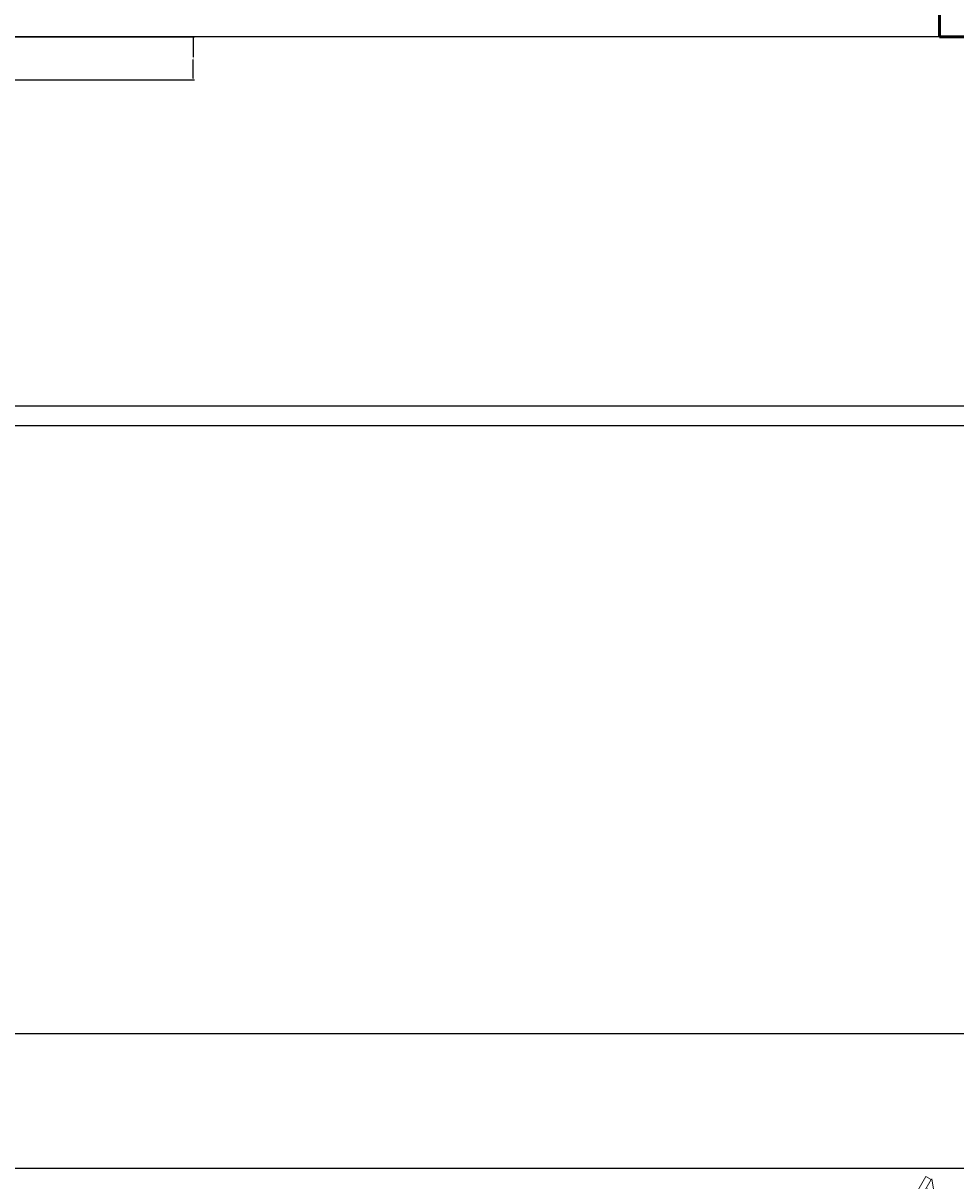
# Model space of a CAD drawing. Units: inches. Extents: x 1865 to 2541, y 1997 to 2759.
# Tile 7 of 11: x 2070 to 2200, y 2405 to 2566. Entities that reach past the tile are written whole.
import ezdxf

# ---------------------------------------------------------------- set-up
doc = ezdxf.new("R2010")
doc.units = ezdxf.units.IN
for name, color, linetype, lineweight in [('A-ANNO-DIMS', 2, 'Continuous', 18), ('A-WALL', 7, 'Continuous', 50), ('DINING TABLE', 120, 'Continuous', 13)]:
    doc.layers.add(name, color=color, linetype=linetype, lineweight=lineweight)
doc.styles.get("Standard").update_dxf_attribs({"font": 'arial.ttf'})
doc.dimstyles.get("Standard").update_dxf_attribs({"dimtxt": 0.18, "dimasz": 0.18, "dimexe": 0.18, "dimexo": 0.0625, "dimgap": 0.09, "dimtad": 0, "dimtih": 1, "dimtoh": 1, "dimdec": 4, "dimzin": 0, "dimdsep": 46, "dimtxsty": 'Standard', "dimcen": 0.09, "dimadec": 0, "dimazin": 0, "dimtfac": 1, "dimtdec": 4, "dimtofl": 0, "dimtmove": 0, "dimatfit": 3, "dimfxl": 1, "dimtolj": 1, "dimtzin": 0, "dimarcsym": 0})

# ---------------------------------------------------------------- blocks, each defined once
blk = doc.blocks.new('A$C45501D90')
for p, q in [((-242.2, 1133.5), (224, 1133.5)), ((-242.2, 1112.8), (-242.2, 1133.5)), ((224, 1112.8), (-242.2, 1112.8)), ((-242.2, 1111.2), (-202.3, 1079.2)), ((-203.9, 1106.4), (-165.6, 1108)), ((-168.8, 1080.8), (-203.9, 1106.4)), ((-165.6, 1108), (-167.2, 1085.6)), ((-156, 1109.6), (-132, 1085.6)), ((-119.3, 1085.6), (-143.2, 1108)), ((-143.2, 1108), (-133.6, 1108)), ((-133.6, 1108), (-122.5, 1098.4)), ((-122.5, 1098.4), (-119.3, 1101.6)), ((-119.3, 1101.6), (-117.7, 1087.2)), ((-108.1, 1109.6), (-84.1, 1085.6)), ((-71.4, 1085.6), (-95.3, 1108)), ((-95.3, 1108), (-85.7, 1108)), ((-85.7, 1108), (-74.6, 1098.4)), ((-74.6, 1098.4), (-71.4, 1101.6)), ((-71.4, 1101.6), (-69.8, 1087.2)), ((-60.2, 1109.6), (-36.2, 1085.6)), ((-23.5, 1085.6), (-47.4, 1108)), ((-47.4, 1108), (-37.8, 1108)), ((-37.8, 1108), (-26.7, 1098.4)), ((-26.7, 1098.4), (-23.5, 1101.6)), ((-23.5, 1101.6), (-21.9, 1087.2)), ((8.5, 1101.6), (6.9, 1087.2)), ((8.5, 1085.6), (32.4, 1108)), ((11.6, 1098.4), (8.5, 1101.6)), ((22.8, 1108), (11.6, 1098.4)), ((45.2, 1109.6), (21.2, 1085.6)), ((32.4, 1108), (22.8, 1108)), ((56.3, 1101.6), (54.8, 1087.2)), ((56.3, 1085.6), (80.3, 1108)), ((59.5, 1098.4), (56.3, 1101.6)), ((70.7, 1108), (59.5, 1098.4)), ((93.1, 1109.6), (69.1, 1085.6)), ((80.3, 1108), (70.7, 1108)), ((104.2, 1101.6), (102.6, 1087.2)), ((104.2, 1085.6), (128.2, 1108)), ((107.4, 1098.4), (104.2, 1101.6)), ((118.6, 1108), (107.4, 1098.4)), ((141, 1109.6), (117, 1085.6)), ((128.2, 1108), (118.6, 1108)), ((188.9, 1106.4), (150.5, 1108)), ((150.5, 1108), (152.1, 1085.6)), ((153.7, 1080.8), (188.9, 1106.4)), ((224, 1112.8), (187.3, 1079.2)), ((224, 1133.5), (224, 1112.8)), ((-197.3, 1061.6), (-238.9, 627.6)), ((-202.3, 1079.2), (-168.8, 1080.8)), ((161.8, 1076.1), (-181.4, 1076.1)), ((-132, 1085.6), (-119.3, 1085.6)), ((-84.1, 1085.6), (-71.4, 1085.6)), ((-36.2, 1085.6), (-23.5, 1085.6)), ((21.2, 1085.6), (8.5, 1085.6)), ((69.1, 1085.6), (56.3, 1085.6)), ((117, 1085.6), (104.2, 1085.6)), ((187.3, 1079.2), (153.7, 1080.8)), ((225.2, 627.8), (177.6, 1061.8)), ((842.6, 766.1), (860.5, 776.5)), ((860.5, 776.5), (1093.6, 372.8)), ((-1102.7, 357), (-869.7, 760.7)), ((-851.7, 750.4), (-1084.8, 346.6)), ((-869.7, 760.7), (-851.7, 750.4)), ((-848.7, 752.3), (-841, 701.8)), ((841.2, 765.3), (833.5, 714.8)), ((1075.7, 362.4), (842.6, 766.1)), ((-863.7, 716.7), (-884.3, 684.4)), ((-859.2, 673.6), (-863.7, 716.7)), ((-841, 701.8), (-859.2, 673.6)), ((820.7, 701.7), (424.1, 520.7)), ((833.5, 714.8), (851.7, 686.6)), ((1012.8, 397.9), (841.2, 695.1)), ((851.7, 686.6), (856.2, 729.8)), ((856.2, 729.8), (876.7, 697.4)), ((876.7, 697.4), (856.6, 687.6)), ((-851, 678.1), (-1022.6, 380.9)), ((-895.4, 665), (-900.2, 656.7)), ((-900.2, 656.7), (-897.5, 642.2)), ((-888.1, 633.1), (-895.4, 665)), ((-890.4, 676.9), (-881.7, 644.2)), ((-884.3, 684.4), (-864.1, 674.6)), ((-431.1, 509), (-830.8, 684.8)), ((882.9, 689.9), (874.2, 657.2)), ((874.2, 657.2), (880.6, 646.1)), ((880.6, 646.1), (887.9, 678)), ((894.4, 654.1), (882.7, 645.5)), ((887.9, 678), (892.7, 669.7)), ((892.7, 669.7), (890, 655.2)), ((890, 655.2), (894.4, 654.1)), ((-919.4, 623.5), (-924.2, 615.2)), ((-924.2, 615.2), (-921.5, 600.8)), ((-912, 591.6), (-919.4, 623.5)), ((-914.4, 635.4), (-905.6, 602.7)), ((-897.5, 642.2), (-901.9, 641.1)), ((-901.9, 641.1), (-890.2, 632.5)), ((-881.7, 644.2), (-888.1, 633.1)), ((906.9, 648.4), (898.1, 615.7)), ((898.1, 615.7), (904.5, 604.6)), ((904.5, 604.6), (911.9, 636.5)), ((918.3, 612.6), (906.7, 604)), ((911.9, 636.5), (916.7, 628.2)), ((916.7, 628.2), (914, 613.8)), ((914, 613.8), (918.3, 612.6)), ((-943.3, 582), (-948.1, 573.8)), ((-948.1, 573.8), (-945.4, 559.3)), ((-936, 550.1), (-943.3, 582)), ((-938.3, 593.9), (-929.6, 561.2)), ((-921.5, 600.8), (-925.8, 599.6)), ((-925.8, 599.6), (-914.2, 591)), ((-905.6, 602.7), (-912, 591.6)), ((-223, 610.1), (209.4, 610.1)), ((930.8, 606.9), (922.1, 574.2)), ((922.1, 574.2), (928.4, 563.1)), ((928.4, 563.1), (935.8, 595.1)), ((942.3, 571.1), (930.6, 562.6)), ((935.8, 595.1), (940.6, 586.8)), ((940.6, 586.8), (937.9, 572.3)), ((937.9, 572.3), (942.3, 571.1)), ((-964.6, 526.1), (-965.7, 530.5)), ((-965.7, 530.5), (-952.5, 524.7)), ((-945.4, 559.3), (-949.8, 558.1)), ((-949.8, 558.1), (-938.1, 549.6)), ((-929.6, 561.2), (-936, 550.1)), ((950.8, 524.4), (944.4, 535.5)), ((944.4, 535.5), (975.7, 525.9)), ((958.2, 543.5), (945, 537.7)), ((957.1, 539.1), (958.2, 543.5)), ((970.9, 534.2), (957.1, 539.1)), ((975.7, 525.9), (970.9, 534.2)), ((-991, 502.7), (-958.3, 511.4)), ((-951.9, 522.5), (-983.2, 512.9)), ((-983.2, 512.9), (-978.5, 521.2)), ((-978.5, 521.2), (-964.6, 526.1)), ((-958.3, 511.4), (-951.9, 522.5)), ((-5.6, 508.7, 90.8), (0.4, 508.7, 90.8)), ((-5.6, 317.7, 90.8), (-5.6, 508.7, 90.8)), ((0.4, 508.7, 90.8), (0.4, 317.7, 90.8)), ((5.8, 317.7, 90.8), (5.8, 508.7, 90.8)), ((5.8, 508.7, 90.8), (11.8, 508.7, 90.8)), ((11.8, 508.7, 90.8), (11.8, 317.7, 90.8)), ((416.9, 498.2), (633.1, 123.7)), ((983.5, 515.7), (950.8, 524.4)), ((968.4, 494), (999.7, 484.4)), ((974.7, 483), (968.4, 494)), ((982.2, 502), (968.9, 496.2)), ((981, 497.6), (982.2, 502)), ((994.9, 492.7), (981, 497.6)), ((999.7, 484.4), (994.9, 492.7)), ((-1015, 461.2), (-982.3, 469.9)), ((-975.9, 481), (-1007.2, 471.4)), ((-1007.2, 471.4), (-1002.4, 479.7)), ((-1002.4, 479.7), (-988.5, 484.6)), ((-988.5, 484.6), (-989.7, 489)), ((-989.7, 489), (-976.5, 483.2)), ((-982.3, 469.9), (-975.9, 481)), ((-639.9, 111.9), (-423.7, 486.4)), ((1007.4, 474.2), (974.7, 483)), ((998.7, 441.5), (992.3, 452.5)), ((992.3, 452.5), (1023.6, 443)), ((1006.1, 460.5), (992.9, 454.7)), ((1005, 456.2), (1006.1, 460.5)), ((1018.8, 451.3), (1005, 456.2)), ((1023.6, 443), (1018.8, 451.3)), ((-1060.1, 376.6), (-1042.3, 410.6)), ((-1042.3, 410.6), (-1023.8, 398.1)), ((-1038.9, 419.7), (-1006.2, 428.5)), ((-999.8, 439.5), (-1031.1, 430)), ((-1031.1, 430), (-1026.3, 438.3)), ((-1026.3, 438.3), (-1012.5, 443.1)), ((-1012.5, 443.1), (-1013.6, 447.5)), ((-1013.6, 447.5), (-1000.4, 441.7)), ((-1006.2, 428.5), (-999.8, 439.5)), ((1031.4, 432.7), (998.7, 441.5)), ((1034.8, 423.6), (1016.3, 411.1)), ((1052.6, 389.6), (1034.8, 423.6)), ((-1020.4, 394.3), (-1060.1, 376.6)), ((-1035.8, 364.4), (-1020.4, 394.3)), ((656.3, 118.9), (1008.4, 377.1)), ((1028.3, 377.5), (1012.9, 407.3)), ((1012.9, 407.3), (1052.6, 389.6)), ((1075.9, 358.8), (1028.3, 377.5)), ((1093.6, 372.8), (1075.7, 362.4)), ((-1084.8, 346.6), (-1102.7, 357)), ((-1083.4, 345.8), (-1035.8, 364.4)), ((-1018, 360), (-663, 106.9)), ((-22.3, 329.1, 90.8), (-22.3, 344.6, 90.8)), ((-22.3, 344.6, 90.8), (-5.6, 344.6, 90.8)), ((-5.6, 329.1, 90.8), (-22.3, 329.1, 90.8)), ((0.4, 344.6, 90.8), (5.8, 344.6, 90.8)), ((5.8, 329.1, 90.8), (0.4, 329.1, 90.8)), ((11.8, 344.6, 90.8), (27.3, 344.6, 90.8)), ((27.3, 329.1, 90.8), (11.8, 329.1, 90.8)), ((27.3, 344.6, 90.8), (27.3, 329.1, 90.8)), ((-175.3, 276.1, 90.8), (-104.8, 293.2, 90.8)), ((-104.8, 293.2, 90.8), (-85.5, 278.4, 90.8)), ((-85.5, 278.4, 90.8), (-52.1, 293.9, 90.8)), ((-52.1, 293.9, 90.8), (9.5, 276.1, 90.8)), ((0.4, 317.7, 90.8), (-5.6, 317.7, 90.8)), ((11.8, 317.7, 90.8), (5.8, 317.7, 90.8)), ((134.3, 288, 90.8), (184.3, 235.5, 90.8)), ((149.7, 213.9, 90.8), (134.3, 288, 90.8)), ((-436.3, 265.3, 90.8), (-433.3, 270.5, 90.8)), ((-270.9, 169.9, 90.8), (-436.3, 265.3, 90.8)), ((-433.3, 270.5, 90.8), (-267.9, 175, 90.8)), ((-430.6, 275.2, 90.8), (-427.6, 280.3, 90.8)), ((-265.2, 179.7, 90.8), (-430.6, 275.2, 90.8)), ((-427.6, 280.3, 90.8), (-262.3, 184.9, 90.8)), ((-103.3, 252.4, 90.8), (-175.3, 276.1, 90.8)), ((-59.5, 246.5, 90.8), (-103.3, 252.4, 90.8)), ((9.5, 276.1, 90.8), (-59.5, 246.5, 90.8)), ((255.2, 161.9, 90.8), (420.6, 257.3, 90.8)), ((423.5, 252.2, 90.8), (258.2, 156.7, 90.8)), ((260.9, 152, 90.8), (426.2, 247.5, 90.8)), ((420.6, 257.3, 90.8), (423.5, 252.2, 90.8)), ((426.2, 247.5, 90.8), (429.2, 242.3, 90.8)), ((-285.5, 198.3, 90.8), (-277.8, 211.7, 90.8)), ((-277.8, 211.7, 90.8), (-264.3, 204, 90.8)), ((-264.3, 204, 90.8), (-272.1, 190.5, 90.8)), ((166.5, 173, 90.8), (149.7, 213.9, 90.8)), ((184.3, 235.5, 90.8), (181.1, 211.4, 90.8)), ((181.1, 211.4, 90.8), (211.3, 190.3, 90.8)), ((429.2, 242.3, 90.8), (263.8, 146.9, 90.8)), ((-302.5, 168.8, 90.8), (-294.2, 183.3, 90.8)), ((-289.1, 161.1, 90.8), (-302.5, 168.8, 90.8)), ((-291.2, 188.5, 90.8), (-288.5, 193.1, 90.8)), ((-280.7, 175.5, 90.8), (-289.1, 161.1, 90.8)), ((-275.1, 185.4, 90.8), (-277.8, 180.7, 90.8)), ((-267.9, 175, 90.8), (-270.9, 169.9, 90.8)), ((-262.3, 184.9, 90.8), (-265.2, 179.7, 90.8)), ((226.7, 128.1, 90.8), (166.5, 173, 90.8)), ((211.3, 190.3, 90.8), (226.7, 128.1, 90.8)), ((256.6, 182, 90.8), (270.1, 189.8, 90.8)), ((265, 167.5, 90.8), (256.6, 182, 90.8)), ((270.1, 189.8, 90.8), (278.4, 175.3, 90.8)), ((281.4, 170.1, 90.8), (284.1, 165.5, 90.8)), ((-273.6, 117.6, 90.8), (-227.4, 162.1, 90.8)), ((-227.4, 162.1, 90.8), (-236.2, 87.5, 90.8)), ((258.2, 156.7, 90.8), (255.2, 161.9, 90.8)), ((263.8, 146.9, 90.8), (260.9, 152, 90.8)), ((270.7, 157.7, 90.8), (268, 162.4, 90.8)), ((281.4, 139.1, 90.8), (273.7, 152.5, 90.8)), ((294.9, 146.8, 90.8), (281.4, 139.1, 90.8)), ((287.1, 160.3, 90.8), (294.9, 146.8, 90.8)), ((-276.8, 80.9, 90.8), (-273.6, 117.6, 90.8)), ((-236.2, 87.5, 90.8), (-263.2, 52.5, 90.8)), ((-319.8, 2.1, 90.8), (-299.3, 71.7, 90.8)), ((-263.2, 52.5, 90.8), (-319.8, 2.1, 90.8)), ((-299.3, 71.7, 90.8), (-276.8, 80.9, 90.8)), ((242.9, -24.6, 90.8), (299.4, 25.9, 90.8)), ((299.4, 25.9, 90.8), (278.9, -43.7, 90.8)), ((215.8, -59.5, 90.8), (242.9, -24.6, 90.8)), ((207, -134.1, 90.8), (215.8, -59.5, 90.8)), ((256.4, -53, 90.8), (253.2, -89.7, 90.8)), ((278.9, -43.7, 90.8), (256.4, -53, 90.8)), ((-656.3, -118.9), (-1008.4, -377.1)), ((-449.6, -214.4, 90.8), (-284.2, -118.9, 90.8)), ((-315.2, -118.9, 90.8), (-301.8, -111.1, 90.8)), ((-307.5, -132.3, 90.8), (-315.2, -118.9, 90.8)), ((-301.8, -111.1, 90.8), (-294, -124.6, 90.8)), ((-284.2, -118.9, 90.8), (-281.2, -124.1, 90.8)), ((-247, -100.1, 90.8), (-186.8, -145, 90.8)), ((-231.7, -162.3, 90.8), (-247, -100.1, 90.8)), ((253.2, -89.7, 90.8), (207, -134.1, 90.8)), ((639.9, -111.9), (423.7, -486.4)), ((1018, -360), (663, -106.9)), ((-416.9, -498.2), (-633.1, -123.7)), ((-281.2, -124.1, 90.8), (-446.6, -219.5, 90.8)), ((-443.9, -224.2, 90.8), (-278.5, -128.7, 90.8)), ((-275.5, -133.9, 90.8), (-440.9, -229.4, 90.8)), ((-301.8, -142.1, 90.8), (-304.5, -137.5, 90.8)), ((-290.4, -161.8, 90.8), (-298.8, -147.3, 90.8)), ((-291, -129.7, 90.8), (-288.3, -134.4, 90.8)), ((-277, -154, 90.8), (-290.4, -161.8, 90.8)), ((-285.4, -139.5, 90.8), (-277, -154, 90.8)), ((-278.5, -128.7, 90.8), (-275.5, -133.9, 90.8)), ((-201.5, -183.4, 90.8), (-231.7, -162.3, 90.8)), ((-186.8, -145, 90.8), (-170.1, -185.9, 90.8)), ((241.9, -156.9, 90.8), (244.9, -151.7, 90.8)), ((407.3, -252.4, 90.8), (241.9, -156.9, 90.8)), ((244, -176, 90.8), (251.7, -162.5, 90.8)), ((244.9, -151.7, 90.8), (410.3, -247.2, 90.8)), ((247.6, -147.1, 90.8), (250.6, -141.9, 90.8)), ((413, -242.5, 90.8), (247.6, -147.1, 90.8)), ((250.6, -141.9, 90.8), (415.9, -237.4, 90.8)), ((254.7, -157.4, 90.8), (257.4, -152.7, 90.8)), ((260.4, -147.6, 90.8), (268.7, -133.1, 90.8)), ((270.8, -160.5, 90.8), (268.1, -165.1, 90.8)), ((268.7, -133.1, 90.8), (282.2, -140.8, 90.8)), ((282.2, -140.8, 90.8), (273.8, -155.3, 90.8)), ((-204.7, -207.6, 90.8), (-201.5, -183.4, 90.8)), ((-170.1, -185.9, 90.8), (-154.7, -260.1, 90.8)), ((257.4, -183.7, 90.8), (244, -176, 90.8)), ((265.2, -170.3, 90.8), (257.4, -183.7, 90.8)), ((-446.6, -219.5, 90.8), (-449.6, -214.4, 90.8)), ((-440.9, -229.4, 90.8), (-443.9, -224.2, 90.8)), ((-154.7, -260.1, 90.8), (-204.7, -207.6, 90.8)), ((-29.8, -248.2, 90.8), (39.2, -218.5, 90.8)), ((39.2, -218.5, 90.8), (83, -224.4, 90.8)), ((83, -224.4, 90.8), (154.9, -248.2, 90.8)), ((415.9, -237.4, 90.8), (413, -242.5, 90.8)), ((31.8, -266, 90.8), (-29.8, -248.2, 90.8)), ((65.2, -250.4, 90.8), (31.8, -266, 90.8)), ((84.4, -265.2, 90.8), (65.2, -250.4, 90.8)), ((154.9, -248.2, 90.8), (84.4, -265.2, 90.8)), ((410.3, -247.2, 90.8), (407.3, -252.4, 90.8)), ((-47.6, -316.6, 90.8), (-47.6, -301.1, 90.8)), ((-47.6, -301.1, 90.8), (-32.1, -301.1, 90.8)), ((-32.1, -316.6, 90.8), (-47.6, -316.6, 90.8)), ((-32.1, -480.7, 90.8), (-32.1, -289.8, 90.8)), ((-32.1, -289.8, 90.8), (-26.1, -289.8, 90.8)), ((-26.1, -289.8, 90.8), (-26.1, -480.7, 90.8)), ((-26.1, -301.1, 90.8), (-20.8, -301.1, 90.8)), ((-20.8, -316.6, 90.8), (-26.1, -316.6, 90.8)), ((-20.8, -480.7, 90.8), (-20.8, -289.8, 90.8)), ((-20.8, -289.8, 90.8), (-14.8, -289.8, 90.8)), ((-14.8, -289.8, 90.8), (-14.8, -480.7, 90.8)), ((-14.8, -301.1, 90.8), (1.9, -301.1, 90.8)), ((1.9, -316.6, 90.8), (-14.8, -316.6, 90.8)), ((1.9, -301.1, 90.8), (1.9, -316.6, 90.8)), ((-1093.6, -372.8), (-1075.7, -362.4)), ((-1075.9, -358.8), (-1028.3, -377.5)), ((-1075.7, -362.4), (-842.6, -766.1)), ((851.7, -750.4), (1084.8, -346.6)), ((1102.7, -357), (869.7, -760.7)), ((1035.8, -364.4), (1020.4, -394.3)), ((1083.4, -345.8), (1035.8, -364.4)), ((1084.8, -346.6), (1102.7, -357)), ((-860.5, -776.5), (-1093.6, -372.8)), ((-1052.6, -389.6), (-1034.8, -423.6)), ((-1012.9, -407.3), (-1052.6, -389.6)), ((-1028.3, -377.5), (-1012.9, -407.3)), ((-1012.8, -397.9), (-841.2, -695.1)), ((851, -678.1), (1022.6, -380.9)), ((1020.4, -394.3), (1060.1, -376.6)), ((1042.3, -410.6), (1023.8, -398.1)), ((1060.1, -376.6), (1042.3, -410.6)), ((-1034.8, -423.6), (-1016.3, -411.1)), ((-1031.4, -432.7), (-998.7, -441.5)), ((-1023.6, -443), (-1018.8, -451.3)), ((-992.3, -452.5), (-1023.6, -443)), ((-998.7, -441.5), (-992.3, -452.5)), ((1006.2, -428.5), (999.8, -439.5)), ((999.8, -439.5), (1031.1, -430)), ((1013.6, -447.5), (1000.4, -441.7)), ((1038.9, -419.7), (1006.2, -428.5)), ((1026.3, -438.3), (1012.5, -443.1)), ((1012.5, -443.1), (1013.6, -447.5)), ((1031.1, -430), (1026.3, -438.3)), ((-1018.8, -451.3), (-1005, -456.2)), ((-1007.4, -474.2), (-974.7, -483)), ((-1006.1, -460.5), (-992.9, -454.7)), ((-1005, -456.2), (-1006.1, -460.5)), ((-968.4, -494), (-999.7, -484.4)), ((-999.7, -484.4), (-994.9, -492.7)), ((-974.7, -483), (-968.4, -494)), ((-26.1, -480.7, 90.8), (-32.1, -480.7, 90.8)), ((-14.8, -480.7, 90.8), (-20.8, -480.7, 90.8)), ((982.3, -469.9), (975.9, -481)), ((975.9, -481), (1007.2, -471.4)), ((989.7, -489), (976.5, -483.2)), ((1015, -461.2), (982.3, -469.9)), ((1002.4, -479.7), (988.5, -484.6)), ((988.5, -484.6), (989.7, -489)), ((1007.2, -471.4), (1002.4, -479.7)), ((-994.9, -492.7), (-981, -497.6)), ((-983.5, -515.7), (-950.8, -524.4)), ((-982.2, -502), (-968.9, -496.2)), ((-981, -497.6), (-982.2, -502)), ((-944.4, -535.5), (-975.7, -525.9)), ((-975.7, -525.9), (-970.9, -534.2)), ((-950.8, -524.4), (-944.4, -535.5)), ((-820.7, -701.7), (-424.1, -520.7)), ((431.1, -509), (830.8, -684.8)), ((958.3, -511.4), (951.9, -522.5)), ((951.9, -522.5), (983.2, -512.9)), ((965.7, -530.5), (952.5, -524.7)), ((991, -502.7), (958.3, -511.4)), ((978.5, -521.2), (964.6, -526.1)), ((964.6, -526.1), (965.7, -530.5)), ((983.2, -512.9), (978.5, -521.2)), ((-970.9, -534.2), (-957.1, -539.1)), ((-958.2, -543.5), (-945, -537.7)), ((-957.1, -539.1), (-958.2, -543.5)), ((-942.3, -571.1), (-930.6, -562.6)), ((-928.4, -563.1), (-935.8, -595.1)), ((-922.1, -574.2), (-928.4, -563.1)), ((929.6, -561.2), (936, -550.1)), ((938.3, -593.9), (929.6, -561.2)), ((936, -550.1), (943.3, -582)), ((949.8, -558.1), (938.1, -549.6)), ((945.4, -559.3), (949.8, -558.1)), ((948.1, -573.8), (945.4, -559.3)), ((-937.9, -572.3), (-942.3, -571.1)), ((-940.6, -586.8), (-937.9, -572.3)), ((-935.8, -595.1), (-940.6, -586.8)), ((-930.8, -606.9), (-922.1, -574.2)), ((-918.3, -612.6), (-906.7, -604)), ((-904.5, -604.6), (-911.9, -636.5)), ((-898.1, -615.7), (-904.5, -604.6)), ((218.9, -611.6), (-213.5, -611.6)), ((223, -610.1), (-209.4, -610.1)), ((905.6, -602.7), (912, -591.6)), ((914.4, -635.4), (905.6, -602.7)), ((912, -591.6), (919.4, -623.5)), ((925.8, -599.6), (914.2, -591)), ((921.5, -600.8), (925.8, -599.6)), ((924.2, -615.2), (921.5, -600.8)), ((943.3, -582), (948.1, -573.8)), ((-914, -613.8), (-918.3, -612.6)), ((-916.7, -628.2), (-914, -613.8)), ((-911.9, -636.5), (-916.7, -628.2)), ((-906.9, -648.4), (-898.1, -615.7)), ((-894.4, -654.1), (-882.7, -645.5)), ((-880.6, -646.1), (-887.9, -678)), ((-874.2, -657.2), (-880.6, -646.1)), ((-229.3, -629.3), (-181.8, -1063.3)), ((-225.2, -627.8), (-177.6, -1061.8)), ((193.2, -1063.1), (234.8, -629.1)), ((197.3, -1061.6), (238.9, -627.6)), ((881.7, -644.2), (888.1, -633.1)), ((890.4, -676.9), (881.7, -644.2)), ((888.1, -633.1), (895.4, -665)), ((901.9, -641.1), (890.2, -632.5)), ((897.5, -642.2), (901.9, -641.1)), ((900.2, -656.7), (897.5, -642.2)), ((919.4, -623.5), (924.2, -615.2)), ((-890, -655.2), (-894.4, -654.1)), ((-892.7, -669.7), (-890, -655.2)), ((-887.9, -678), (-892.7, -669.7)), ((-882.9, -689.9), (-874.2, -657.2)), ((-876.7, -697.4), (-856.6, -687.6)), ((-851.7, -686.6), (-856.2, -729.8)), ((-833.5, -714.8), (-851.7, -686.6)), ((841, -701.8), (859.2, -673.6)), ((859.2, -673.6), (863.7, -716.7)), ((863.7, -716.7), (884.3, -684.4)), ((884.3, -684.4), (864.1, -674.6)), ((895.4, -665), (900.2, -656.7)), ((-856.2, -729.8), (-876.7, -697.4)), ((-841.2, -765.3), (-833.5, -714.8)), ((848.7, -752.3), (841, -701.8)), ((-842.6, -766.1), (-860.5, -776.5)), ((869.7, -760.7), (851.7, -750.4)), ((-231.3, -1112.7), (-191.4, -1080.8)), ((-227.2, -1111.2), (-187.3, -1079.2)), ((-157.9, -1082.4), (-193, -1107.9)), ((-191.4, -1080.8), (-157.9, -1082.4)), ((-153.7, -1080.8), (-188.9, -1106.4)), ((-187.3, -1079.2), (-153.7, -1080.8)), ((-165.9, -1077.6), (177.3, -1077.6)), ((-161.8, -1076.1), (181.4, -1076.1)), ((-154.7, -1109.5), (-156.3, -1087.1)), ((-150.5, -1108), (-152.1, -1085.6)), ((-145.1, -1111.1), (-121.1, -1087.1)), ((-141, -1109.6), (-117, -1085.6)), ((-108.4, -1087.1), (-132.3, -1109.5)), ((-104.2, -1085.6), (-128.2, -1108)), ((-122.7, -1109.5), (-111.6, -1099.9)), ((-121.1, -1087.1), (-108.4, -1087.1)), ((-118.6, -1108), (-107.4, -1098.4)), ((-117, -1085.6), (-104.2, -1085.6)), ((-111.6, -1099.9), (-108.4, -1103.1)), ((-108.4, -1103.1), (-106.8, -1088.7)), ((-107.4, -1098.4), (-104.2, -1101.6)), ((-104.2, -1101.6), (-102.6, -1087.2)), ((-97.2, -1111.1), (-73.2, -1087.1)), ((-93.1, -1109.6), (-69.1, -1085.6)), ((-60.5, -1087.1), (-84.4, -1109.5)), ((-56.3, -1085.6), (-80.3, -1108)), ((-74.8, -1109.5), (-63.7, -1099.9)), ((-73.2, -1087.1), (-60.5, -1087.1)), ((-70.7, -1108), (-59.5, -1098.4)), ((-69.1, -1085.6), (-56.3, -1085.6)), ((-63.7, -1099.9), (-60.5, -1103.1)), ((-60.5, -1103.1), (-58.9, -1088.7)), ((-59.5, -1098.4), (-56.3, -1101.6)), ((-56.3, -1101.6), (-54.8, -1087.2)), ((-49.3, -1111.1), (-25.3, -1087.1)), ((-45.2, -1109.6), (-21.2, -1085.6)), ((-12.6, -1087.1), (-36.5, -1109.5)), ((-8.5, -1085.6), (-32.4, -1108)), ((-26.9, -1109.5), (-15.8, -1099.9)), ((-25.3, -1087.1), (-12.6, -1087.1)), ((-22.8, -1108), (-11.6, -1098.4)), ((-21.2, -1085.6), (-8.5, -1085.6)), ((-15.8, -1099.9), (-12.6, -1103.1)), ((-12.6, -1103.1), (-11, -1088.7)), ((-11.6, -1098.4), (-8.5, -1101.6)), ((-8.5, -1101.6), (-6.9, -1087.2)), ((19.4, -1103.1), (17.8, -1088.7)), ((19.4, -1087.1), (43.3, -1109.5)), ((32.1, -1087.1), (19.4, -1087.1)), ((22.6, -1099.9), (19.4, -1103.1)), ((23.5, -1101.6), (21.9, -1087.2)), ((33.7, -1109.5), (22.6, -1099.9)), ((23.5, -1085.6), (47.4, -1108)), ((36.2, -1085.6), (23.5, -1085.6)), ((26.7, -1098.4), (23.5, -1101.6)), ((37.8, -1108), (26.7, -1098.4)), ((56.1, -1111.1), (32.1, -1087.1)), ((60.2, -1109.6), (36.2, -1085.6)), ((67.3, -1103.1), (65.7, -1088.7)), ((67.3, -1087.1), (91.2, -1109.5)), ((80, -1087.1), (67.3, -1087.1)), ((70.4, -1099.9), (67.3, -1103.1)), ((71.4, -1101.6), (69.8, -1087.2)), ((81.6, -1109.5), (70.4, -1099.9)), ((71.4, -1085.6), (95.3, -1108)), ((84.1, -1085.6), (71.4, -1085.6)), ((74.6, -1098.4), (71.4, -1101.6)), ((85.7, -1108), (74.6, -1098.4)), ((104, -1111.1), (80, -1087.1)), ((108.1, -1109.6), (84.1, -1085.6)), ((115.1, -1103.1), (113.6, -1088.7)), ((115.1, -1087.1), (139.1, -1109.5)), ((127.9, -1087.1), (115.1, -1087.1)), ((118.3, -1099.9), (115.1, -1103.1)), ((119.3, -1101.6), (117.7, -1087.2)), ((129.5, -1109.5), (118.3, -1099.9)), ((119.3, -1085.6), (143.2, -1108)), ((132, -1085.6), (119.3, -1085.6)), ((122.5, -1098.4), (119.3, -1101.6)), ((133.6, -1108), (122.5, -1098.4)), ((151.9, -1111.1), (127.9, -1087.1)), ((156, -1109.6), (132, -1085.6)), ((161.4, -1109.5), (163, -1087.1)), ((198.2, -1080.8), (164.6, -1082.4)), ((164.6, -1082.4), (199.8, -1107.9)), ((165.6, -1108), (167.2, -1085.6)), ((202.3, -1079.2), (168.8, -1080.8)), ((168.8, -1080.8), (203.9, -1106.4)), ((238.1, -1112.7), (198.2, -1080.8)), ((242.2, -1111.2), (202.3, -1079.2)), ((-228.1, -1114.3), (238.1, -1114.3)), ((-228.1, -1135), (-228.1, -1114.3)), ((238.1, -1135), (-228.1, -1135)), ((-224, -1112.8), (242.2, -1112.8)), ((-224, -1133.5), (-224, -1112.8)), ((242.2, -1133.5), (-224, -1133.5)), ((-193, -1107.9), (-154.7, -1109.5)), ((-188.9, -1106.4), (-150.5, -1108)), ((-132.3, -1109.5), (-122.7, -1109.5)), ((-128.2, -1108), (-118.6, -1108)), ((-84.4, -1109.5), (-74.8, -1109.5)), ((-80.3, -1108), (-70.7, -1108)), ((-36.5, -1109.5), (-26.9, -1109.5)), ((-32.4, -1108), (-22.8, -1108)), ((43.3, -1109.5), (33.7, -1109.5)), ((47.4, -1108), (37.8, -1108)), ((91.2, -1109.5), (81.6, -1109.5)), ((95.3, -1108), (85.7, -1108)), ((139.1, -1109.5), (129.5, -1109.5)), ((143.2, -1108), (133.6, -1108)), ((199.8, -1107.9), (161.4, -1109.5)), ((203.9, -1106.4), (165.6, -1108)), ((238.1, -1114.3), (238.1, -1135)), ((242.2, -1112.8), (242.2, -1133.5))]:
    blk.add_line(p, q)
for centre, radius in [((0, 0), 537), ((0, 0), 527), ((-94.8, 394.7, 90.8), 61.3), ((96.9, 390, 90.8), 56.9), ((95.5, 390.7, 90.8), 29.4), ((-282.3, 294.7, 90.8), 56.9), ((277.2, 277.6, 90.8), 61.3), ((-283.5, 293.9, 90.8), 29.4), ((-382.1, 131.1, 90.8), 61.3), ((369, 109.3, 90.8), 56.9), ((368.9, 110.8, 90.8), 29.4), ((-389.3, -81.3, 90.8), 56.9), ((-389.2, -82.8, 90.8), 29.4), ((361.8, -103.1, 90.8), 61.3), ((-297.5, -249.6, 90.8), 61.3), ((261.9, -266.7, 90.8), 56.9), ((263.2, -265.9, 90.8), 29.4), ((-117.2, -362, 90.8), 56.9), ((74.4, -366.7, 90.8), 61.3), ((-115.9, -362.7, 90.8), 29.4)]:
    blk.add_circle(centre, radius)
for centre, radius, start, end in [((-181.4, 1060.1), 16, 90, 174.5199), ((161.8, 1060.1), 16, 6.2572, 90), ((827.4, 687.1), 16, 30, 114.5199), ((-837.2, 670.1), 16, 66.2572, 150), ((-223, 626.1), 16, 174.5199, 270), ((209.4, 626.1), 16, 270, 6.2572), ((-437.5, 494.4), 16, 330, 66.2572), ((430.7, 506.2), 16, 114.5199, 210), ((-1008.8, 373), 16, 150, 234.5199), ((999, 389.9), 16, 306.2572, 30), ((-77.3, 270.2, 90.8), 44.6, 25.8558, 153.3359), ((-77.3, 270.2, 90.8), 44.6, 195.9338, 342.9389), ((178.1, 200.3, 90.8), 44.6, 325.8558, 93.3359), ((178.1, 200.3, 90.8), 44.6, 135.9338, 282.9389), ((-265.7, 83.9, 90.8), 44.6, 85.8558, 213.3359), ((646.9, 131.7), 16, 210, 306.2572), ((-653.7, 119.9), 16, 234.5199, 330), ((-265.7, 83.9, 90.8), 44.6, 255.9338, 42.9389), ((245.3, -55.9, 90.8), 44.6, 75.9338, 222.9389), ((245.3, -55.9, 90.8), 44.6, 265.8558, 33.3359), ((-646.9, -131.7), 16, 30, 126.2572), ((653.7, -119.9), 16, 54.5199, 150), ((-198.5, -172.3, 90.8), 44.6, 145.8558, 273.3359), ((-198.5, -172.3, 90.8), 44.6, 315.9338, 102.9389), ((57, -242.2, 90.8), 44.6, 15.9338, 162.9389), ((57, -242.2, 90.8), 44.6, 205.8558, 333.3359), ((1008.8, -373), 16, 330, 54.5199), ((-999, -389.9), 16, 126.2572, 210), ((437.5, -494.4), 16, 150, 246.2572), ((-430.7, -506.2), 16, 294.5199, 30), ((-213.5, -627.6), 16, 90, 186.2572), ((-209.4, -626.1), 16, 90, 186.2572), ((218.9, -627.6), 16, 354.5199, 90), ((223, -626.1), 16, 354.5199, 90), ((837.2, -670.1), 16, 246.2572, 330), ((-827.4, -687.1), 16, 210, 294.5199), ((-165.9, -1061.6), 16, 186.2572, 270), ((-161.8, -1060.1), 16, 186.2572, 270), ((177.3, -1061.6), 16, 270, 354.5199), ((181.4, -1060.1), 16, 270, 354.5199)]:
    blk.add_arc(centre, radius, start, end)
blk = doc.blocks.new('*D41')
at = {"layer": 'A-ANNO-DIMS', "color": 0, "lineweight": -2, "transparency": 16777216}
for p, q in [((2503.31, 2721.45), (2540.92, 2721.45)), ((2540.74, 2721.27), (2540.74, 2378.49)), ((2540.74, 2035.35), (2540.74, 2378.13)), ((2136.19, 2035.17), (2540.92, 2035.17))]:
    blk.add_line(p, q, dxfattribs=at)
at = {"layer": 'A-ANNO-DIMS', "color": 0, "transparency": 16777216}
for points in [[(2540.71, 2721.27), (2540.77, 2721.27), (2540.74, 2721.45)], [(2540.71, 2035.35), (2540.77, 2035.35), (2540.74, 2035.17)]]:
    blk.add_solid(points, dxfattribs=at)
at = {"layer": 'Defpoints', "color": 0, "transparency": 16777216}
for p in [(2503.24, 2721.45), (2136.13, 2035.17), (2540.74, 2035.17)]:
    blk.add_point(p, dxfattribs=at)
at = {"layer": 'A-ANNO-DIMS', "color": 0, "transparency": 16777216, "insert": (2540.74, 2378.31), "char_height": 0.18, "attachment_point": 5}
blk.add_mtext('\\A1;686.3', dxfattribs=at)
blk = doc.blocks.new('*D63')
at = {"layer": 'A-ANNO-DIMS', "color": 0, "lineweight": -2, "transparency": 16777216}
for p, q in [((2404.18, 2563.95), (1865.56, 2563.95)), ((1865.74, 2563.77), (1865.74, 2538.51)), ((1865.74, 2512.9), (1865.74, 2538.15)), ((2404.18, 2512.72), (1865.56, 2512.72))]:
    blk.add_line(p, q, dxfattribs=at)
at = {"layer": 'A-ANNO-DIMS', "color": 0, "transparency": 16777216}
for points in [[(1865.71, 2563.77), (1865.77, 2563.77), (1865.74, 2563.95)], [(1865.71, 2512.9), (1865.77, 2512.9), (1865.74, 2512.72)]]:
    blk.add_solid(points, dxfattribs=at)
at = {"layer": 'Defpoints', "color": 0, "transparency": 16777216}
for p in [(2404.24, 2563.95), (1865.74, 2512.72), (2404.24, 2512.72)]:
    blk.add_point(p, dxfattribs=at)
at = {"layer": 'A-ANNO-DIMS', "color": 0, "transparency": 16777216, "insert": (1865.74, 2538.33), "char_height": 0.18, "attachment_point": 5}
blk.add_mtext('\\A1;51.23', dxfattribs=at)
blk = doc.blocks.new('*D66')
at = {"layer": 'A-ANNO-DIMS', "color": 0, "lineweight": -2, "transparency": 16777216}
for p, q in [((2408.32, 2425.66), (1865.56, 2425.66)), ((1865.74, 2425.48), (1865.74, 2416.48)), ((1865.74, 2407.13), (1865.74, 2416.12)), ((2408.32, 2406.95), (1865.56, 2406.95))]:
    blk.add_line(p, q, dxfattribs=at)
at = {"layer": 'A-ANNO-DIMS', "color": 0, "transparency": 16777216}
for points in [[(1865.71, 2425.48), (1865.77, 2425.48), (1865.74, 2425.66)], [(1865.71, 2407.13), (1865.77, 2407.13), (1865.74, 2406.95)]]:
    blk.add_solid(points, dxfattribs=at)
at = {"layer": 'Defpoints', "color": 0, "transparency": 16777216}
for p in [(2408.38, 2425.66), (1865.74, 2406.95), (2408.38, 2406.95)]:
    blk.add_point(p, dxfattribs=at)
at = {"layer": 'A-ANNO-DIMS', "color": 0, "transparency": 16777216, "insert": (1865.74, 2416.3), "char_height": 0.18, "attachment_point": 5}
blk.add_mtext('\\A1;18.706', dxfattribs=at)
blk = doc.blocks.new('*D67')
at = {"layer": 'A-ANNO-DIMS', "color": 0, "lineweight": -2, "transparency": 16777216}
for p, q in [((2475.89, 2509.99), (1865.56, 2509.99)), ((1865.74, 2509.81), (1865.74, 2468)), ((1865.74, 2425.84), (1865.74, 2467.64)), ((2475.89, 2425.66), (1865.56, 2425.66))]:
    blk.add_line(p, q, dxfattribs=at)
at = {"layer": 'A-ANNO-DIMS', "color": 0, "transparency": 16777216}
for points in [[(1865.71, 2509.81), (1865.77, 2509.81), (1865.74, 2509.99)], [(1865.71, 2425.84), (1865.77, 2425.84), (1865.74, 2425.66)]]:
    blk.add_solid(points, dxfattribs=at)
at = {"layer": 'Defpoints', "color": 0, "transparency": 16777216}
for p in [(1865.74, 2509.99), (2475.95, 2509.99), (2475.95, 2425.66)]:
    blk.add_point(p, dxfattribs=at)
at = {"layer": 'A-ANNO-DIMS', "color": 0, "transparency": 16777216, "insert": (1865.74, 2467.82), "char_height": 0.18, "attachment_point": 5}
blk.add_mtext('\\A1;84.33', dxfattribs=at)
blk = doc.blocks.new('*D79')
at = {"layer": 'A-ANNO-DIMS', "color": 0, "lineweight": -2, "transparency": 16777216}
for p, q in [((2056.31, 2563.95), (2093.92, 2563.95)), ((2093.74, 2563.77), (2093.74, 2561.13)), ((2093.74, 2558.13), (2093.74, 2560.77)), ((2056.31, 2557.95), (2093.92, 2557.95))]:
    blk.add_line(p, q, dxfattribs=at)
at = {"layer": 'A-ANNO-DIMS', "color": 0, "transparency": 16777216}
for points in [[(2093.71, 2563.77), (2093.77, 2563.77), (2093.74, 2563.95)], [(2093.71, 2558.13), (2093.77, 2558.13), (2093.74, 2557.95)]]:
    blk.add_solid(points, dxfattribs=at)
at = {"layer": 'Defpoints', "color": 0, "transparency": 16777216}
for p in [(2056.24, 2563.95), (2056.24, 2557.95), (2093.74, 2557.95)]:
    blk.add_point(p, dxfattribs=at)
at = {"layer": 'A-ANNO-DIMS', "color": 0, "transparency": 16777216, "insert": (2093.74, 2560.95), "char_height": 0.18, "attachment_point": 5}
blk.add_mtext('\\A1;6', dxfattribs=at)

msp = doc.modelspace()

# ---------------------------------------------------------------- linework, layer by layer
at = {"layer": 'A-WALL'}
for p in [(2197.243, 2568.4494), (2207.743, 2563.9494)]:
    msp.add_line(p, (2197.243, 2563.9494), dxfattribs=at)

# ---------------------------------------------------------------- block references
at = {"layer": 'DINING TABLE', "xscale": 0.0393700787401575, "yscale": 0.0393700787401575, "zscale": 0.0393700787401575}
msp.add_blockref('A$C45501D90', (2229.6028, 2375.915, -3.5735), dxfattribs=at)

# ---------------------------------------------------------------- dimensions: what is measured, and where the dimension line sits
at = {"layer": 'A-ANNO-DIMS'}
for base, p1, p2, angle, override, picture, middle in [((2540.743, 2035.1708), (2503.243, 2721.4494), (2136.13, 2035.1708), 90, {"dimdec": 1, "dimlfac": 1, "dimrnd": 0, "dimzin": 0, "dimdsep": 46, "dimlunit": 2}, '*D41', (2540.743, 2378.3101)), ((1865.743, 2512.7166), (2404.243, 2563.9494), (2404.243, 2512.7166), 90, {"dimdec": 2, "dimlfac": 1, "dimrnd": 0, "dimzin": 0, "dimdsep": 46, "dimlunit": 2}, '*D63', (1865.743, 2538.333)), ((2093.743, 2557.9494), (2056.243, 2563.9494), (2056.243, 2557.9494), 270, {"dimdec": 0, "dimlfac": 1, "dimrnd": 0, "dimzin": 0, "dimdsep": 46, "dimlunit": 2}, '*D79', (2093.743, 2560.9494)), ((1865.743, 2509.9875), (2475.9518, 2425.6552), (2475.9518, 2509.9875), 90, {"dimdec": 2, "dimlfac": 1, "dimrnd": 0, "dimzin": 0, "dimdsep": 46, "dimlunit": 2}, '*D67', (1865.743, 2467.8214)), ((1865.743, 2406.9494), (2408.3779, 2425.6552), (2408.3779, 2406.9494), 90, {"dimdec": 3, "dimlfac": 1, "dimrnd": 0, "dimzin": 0, "dimdsep": 46, "dimlunit": 2}, '*D66', (1865.743, 2416.3023))]:
    dim = msp.add_linear_dim(base=base, p1=p1, p2=p2, angle=angle, dimstyle='Standard', override=override, dxfattribs=at)
    dim.commit()
    dim.dimension.update_dxf_attribs({"geometry": picture, "text_midpoint": middle})

doc.saveas('drawing.dxf')
